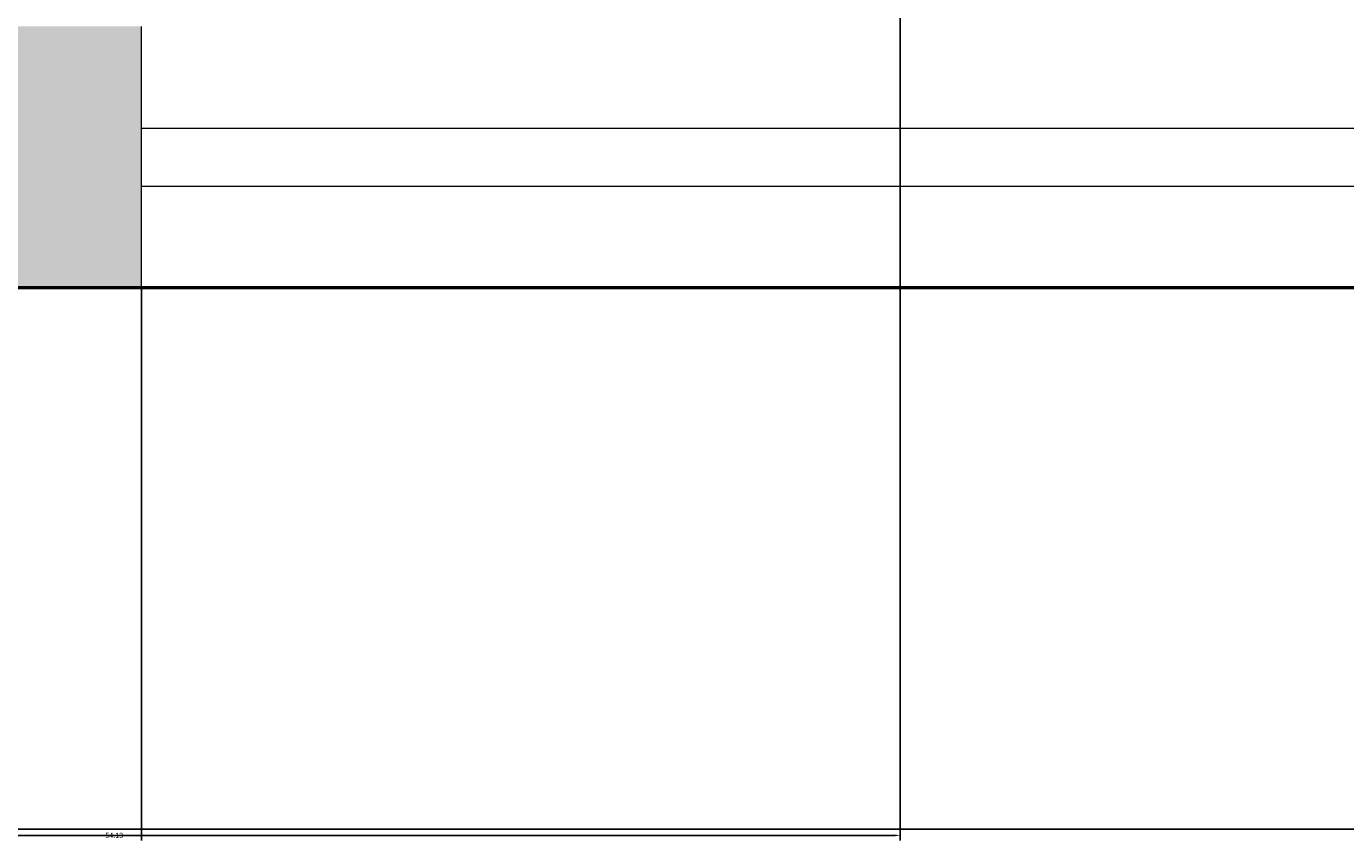
# Model space of a CAD drawing. Units: inches. Extents: x 2231 to 2461, y 2045 to 2455.
# Tile 18 of 95: x 2365 to 2410, y 2045 to 2073. Entities that reach past the tile are written whole.
import ezdxf

# ---------------------------------------------------------------- set-up
doc = ezdxf.new("R2010")
doc.units = ezdxf.units.IN
for name, color, linetype, lineweight in [('A-ANNO-DIMS', 2, 'Continuous', 18), ('A-GLAZ', 4, 'Continuous', 18), ('A-WALL', 7, 'Continuous', 50)]:
    doc.layers.add(name, color=color, linetype=linetype, lineweight=lineweight)
doc.layers.add('A-WALL-PATT', color=18, linetype='Continuous', lineweight=13, true_color=0x000000)
doc.styles.get("Standard").update_dxf_attribs({"font": 'arial.ttf'})
doc.dimstyles.get("Standard").update_dxf_attribs({"dimtxt": 0.18, "dimasz": 0.18, "dimexe": 0.18, "dimexo": 0.0625, "dimgap": 0.09, "dimtad": 0, "dimtih": 1, "dimtoh": 1, "dimdec": 4, "dimzin": 0, "dimdsep": 46, "dimtxsty": 'Standard', "dimcen": 0.09, "dimadec": 0, "dimazin": 0, "dimtfac": 1, "dimtdec": 4, "dimtofl": 0, "dimtmove": 0, "dimatfit": 3, "dimfxl": 1, "dimtolj": 1, "dimtzin": 0, "dimarcsym": 0})

# ---------------------------------------------------------------- blocks, each defined once
blk = doc.blocks.new('WIN-48IN')
for p, q in [((0, 0), (0, 9)), ((0, 5.5), (48, 5.5)), ((0, 3.5), (48, 3.5))]:
    blk.add_line(p, q)
blk = doc.blocks.new('*D33')
at = {"layer": 'A-ANNO-DIMS', "color": 0, "lineweight": -2, "transparency": 16777216}
for p, q in [((2249.794, 2063.77), (2249.794, 2045.02)), ((2441.794, 2063.77), (2441.794, 2045.02)), ((2249.974, 2045.2), (2345.514, 2045.2)), ((2441.614, 2045.2), (2346.073, 2045.2))]:
    blk.add_line(p, q, dxfattribs=at)
at = {"layer": 'A-ANNO-DIMS', "color": 0, "transparency": 16777216}
for points in [[(2249.974, 2045.23), (2249.974, 2045.17), (2249.794, 2045.2)], [(2441.614, 2045.23), (2441.614, 2045.17), (2441.794, 2045.2)]]:
    blk.add_solid(points, dxfattribs=at)
at = {"layer": 'Defpoints', "color": 0, "transparency": 16777216}
for p in [(2249.794, 2063.833), (2441.794, 2063.833), (2249.794, 2045.2)]:
    blk.add_point(p, dxfattribs=at)
at = {"layer": 'A-ANNO-DIMS', "color": 0, "transparency": 16777216, "insert": (2345.794, 2045.2), "char_height": 0.18, "attachment_point": 5}
blk.add_mtext('\\A1;192', dxfattribs=at)
blk = doc.blocks.new('*D46')
at = {"layer": 'A-ANNO-DIMS', "color": 0, "lineweight": -2, "transparency": 16777216}
for p, q in [((2330.74, 2063.77), (2330.74, 2044.803)), ((2368.664, 2063.77), (2368.664, 2044.803)), ((2330.92, 2044.983), (2349.239, 2044.983)), ((2368.484, 2044.983), (2350.165, 2044.983))]:
    blk.add_line(p, q, dxfattribs=at)
at = {"layer": 'A-ANNO-DIMS', "color": 0, "transparency": 16777216}
for points in [[(2330.92, 2045.013), (2330.92, 2044.953), (2330.74, 2044.983)], [(2368.484, 2045.013), (2368.484, 2044.953), (2368.664, 2044.983)]]:
    blk.add_solid(points, dxfattribs=at)
at = {"layer": 'Defpoints', "color": 0, "transparency": 16777216}
for p in [(2330.74, 2063.833), (2368.664, 2063.833), (2368.664, 2044.983)]:
    blk.add_point(p, dxfattribs=at)
at = {"layer": 'A-ANNO-DIMS', "color": 0, "transparency": 16777216, "insert": (2349.702, 2044.983), "char_height": 0.18, "attachment_point": 5}
blk.add_mtext('\\A1;37.924', dxfattribs=at)
blk = doc.blocks.new('*D69')
at = {"layer": 'A-ANNO-DIMS', "color": 0, "lineweight": -2, "transparency": 16777216}
for p, q in [((2340.667, 2189.285), (2340.667, 2044.803)), ((2394.794, 2186.77), (2394.794, 2044.803)), ((2340.847, 2044.983), (2367.337, 2044.983)), ((2394.614, 2044.983), (2368.124, 2044.983))]:
    blk.add_line(p, q, dxfattribs=at)
at = {"layer": 'A-ANNO-DIMS', "color": 0, "transparency": 16777216}
for points in [[(2340.847, 2045.013), (2340.847, 2044.953), (2340.667, 2044.983)], [(2394.614, 2045.013), (2394.614, 2044.953), (2394.794, 2044.983)]]:
    blk.add_solid(points, dxfattribs=at)
at = {"layer": 'Defpoints', "color": 0, "transparency": 16777216}
for p in [(2340.667, 2189.348), (2394.794, 2186.833), (2394.794, 2044.983)]:
    blk.add_point(p, dxfattribs=at)
at = {"layer": 'A-ANNO-DIMS', "color": 0, "transparency": 16777216, "insert": (2367.73, 2044.983), "char_height": 0.18, "attachment_point": 5}
blk.add_mtext('\\A1;54.13', dxfattribs=at)

msp = doc.modelspace()

# ---------------------------------------------------------------- hatches: boundary and pattern name
at = {"layer": 'A-WALL-PATT'}
h = msp.add_hatch(color=256, dxfattribs=at)
h.dxf.hatch_style = 1
h.paths.add_polyline_path([(2441.7935, 2269.1535), (2432.7935, 2269.1535), (2432.7935, 2186.8328), (2396.7935, 2186.8328), (2396.7935, 2286.8328), (2394.7935, 2286.8328), (2394.7935, 2186.8328), (2334.7935, 2186.8328), (2334.7935, 2182.8328), (2432.7935, 2182.8328), (2432.7935, 2072.8328), (2416.6639, 2072.8328), (2416.6639, 2063.8328), (2441.7935, 2063.8328)])
h.paths.add_polyline_path([(2368.6639, 2072.8328), (2367.04, 2072.8328), (2330.7942, 2072.8328), (2330.7397, 2063.8328), (2368.6639, 2063.8328)])
h.paths.add_polyline_path([(2300.7392, 2068.3328), (2300.7392, 2072.8328), (2298.7935, 2072.8328), (2294.7935, 2072.8328), (2258.7935, 2072.8328), (2258.7935, 2120.8328), (2294.7935, 2120.8328), (2298.7935, 2120.8328), (2298.7935, 2128.8328), (2294.7935, 2128.8328), (2294.7935, 2124.8328), (2258.7935, 2124.8328), (2258.7935, 2182.8328), (2294.7935, 2182.8328), (2294.7935, 2174.8328), (2298.7935, 2174.8328), (2298.7935, 2182.8328), (2304.7935, 2182.8328), (2304.7935, 2186.8328), (2258.7935, 2186.8328), (2258.7935, 2221.999), (2249.7935, 2221.999), (2249.7935, 2063.8328), (2300.7392, 2063.8328)])
h.paths.add_polyline_path([(2391.9338, 2435.8328), (2333.82, 2435.8328), (2333.82, 2426.8328), (2368.7935, 2426.8328), (2368.7935, 2374.9508), (2368.7935, 2370.8328), (2372.3935, 2370.8328), (2372.7935, 2370.8328), (2372.7935, 2426.8328), (2391.9338, 2426.8328)])
h.paths.add_polyline_path([(2441.7935, 2435.8328), (2415.9338, 2435.8328), (2415.9338, 2426.8328), (2432.7935, 2426.8328), (2432.7935, 2334.8328), (2372.7935, 2334.8328), (2372.7935, 2346.8328), (2368.7935, 2346.8328), (2368.7935, 2306.8328), (2360.7935, 2306.8328), (2360.7935, 2302.8328), (2368.7935, 2302.8328), (2372.7935, 2302.8328), (2372.7935, 2330.8328), (2432.7935, 2330.8328), (2432.7935, 2317.1535), (2441.7935, 2317.1535)])
h.paths.add_polyline_path([(2285.82, 2435.8328), (2249.7935, 2435.8328), (2249.7935, 2269.999), (2258.7935, 2269.999), (2258.7935, 2302.8328), (2318.8168, 2302.8328), (2330.7935, 2302.8328), (2330.7935, 2306.8328), (2258.7935, 2306.8328), (2258.7935, 2426.8328), (2285.82, 2426.8328)])

# ---------------------------------------------------------------- linework, layer by layer
at = {"layer": 'A-WALL'}
msp.add_lwpolyline([(2300.7392, 2063.8328), (2249.7935, 2063.8328), (2249.7935, 2435.8328), (2441.7935, 2435.8328), (2441.7935, 2063.8328), (2330.7397, 2063.8328)], dxfattribs=at)

# ---------------------------------------------------------------- block references
at = {"layer": 'A-GLAZ'}
msp.add_blockref('WIN-48IN', (2368.6639, 2063.833), dxfattribs=at)

# ---------------------------------------------------------------- dimensions: what is measured, and where the dimension line sits
at = {"layer": 'A-ANNO-DIMS'}
for base, p1, p2, override, picture, middle in [((2394.7935, 2044.9825), (2340.6673, 2189.3477), (2394.7935, 2186.8328), {"dimdec": 2, "dimlfac": 1, "dimrnd": 0, "dimzin": 0, "dimdsep": 46, "dimlunit": 2}, '*D69', (2367.7304, 2044.9825)), ((2368.6639, 2044.9825), (2330.7397, 2063.8328), (2368.6639, 2063.8328), {"dimdec": 3, "dimlfac": 1, "dimrnd": 0, "dimzin": 0, "dimdsep": 46, "dimlunit": 2}, '*D46', (2349.7018, 2044.9825))]:
    dim = msp.add_linear_dim(base=base, p1=p1, p2=p2, dimstyle='Standard', override=override, dxfattribs=at)
    dim.commit()
    dim.dimension.update_dxf_attribs({"geometry": picture, "text_midpoint": middle})
dim = msp.add_linear_dim(base=(2249.7935, 2045.2003), p1=(2441.7935, 2063.8328), p2=(2249.7935, 2063.8328), angle=180, dimstyle='Standard', override={"dimdec": 0, "dimlfac": 1, "dimrnd": 0, "dimzin": 0, "dimdsep": 46, "dimlunit": 2}, dxfattribs=at)
dim.commit()
dim.dimension.update_dxf_attribs({"geometry": '*D33', "text_midpoint": (2345.7935, 2045.2003)})

doc.saveas('drawing.dxf')
